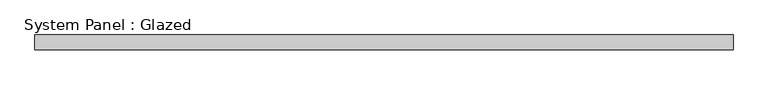
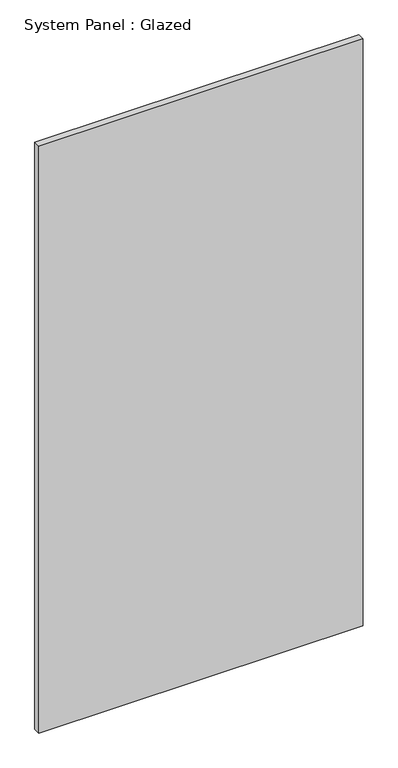
"""IFC4 building model written with IfcOpenShell, lengths in millimetres: plate geometry, System Panel : Glazed."""

from ifc_helpers import new_model, si_unit, origin, origin_with_axes, place, context, project, spatial, polyline, outline, extrude, source, transform, mapped, element, save


def system_panel_glazed_4219beb1(model_context):
    return source(origin(), model_context, "Body", "SweptSolid", [
        extrude(outline(polyline([(604.3083333, 19.05), (-604.3083333, 19.05), (-604.3083333, 44.45), (604.3083333, 44.45), (604.3083333, 19.05)])), origin_with_axes(), (0.0, 0.0, 1.0), 2311.4),
    ])


if __name__ == "__main__":
    model = new_model("IFC4")
    model_context = context("Model", 3, world=origin())
    ifc_project = project(units=[si_unit("LENGTHUNIT", "METRE", prefix="MILLI")], contexts=[model_context])
    site = spatial("IfcSite", under=ifc_project)
    building = spatial("IfcBuilding", under=site)
    placement = place(None, origin())
    system_panel_glazed_shape = system_panel_glazed_4219beb1(model_context)
    element("IfcPlate", 1, ObjectType="System Panel : Glazed", at=placement, inside=building, context=model_context, shape_type="MappedRepresentation", body=[
        mapped(system_panel_glazed_shape, transform((0.0, 0.0, 0.0), x_axis=(1.0, 0.0, 0.0), y_axis=(0.0, 1.0, 0.0), z_axis=(0.0, 0.0, 1.0))),
    ])
    save(model, "model.ifc")

# Revit data of these elements
# Type "System Panel : Glazed"
#   Construction Type Id = "GSP4R"
#   Analytic Construction = "1/8 in Pilkington single glazing"
#   Visual Light Transmittance = 0.9
#   Solar Heat Gain Coefficient = 0.86
#   Heat Transfer Coefficient (U) = 1.18115 BTU/(h·ft²·°F)
# Element 1 (IfcPlate, "System Panel : Glazed")
#   Materials on its faces: "Glass"
# Materials
#   "Glass": class "Glass", colour RGB 0 128 192, transparency 0.75, Description = "Soda Lime Glass", Cost = 0
